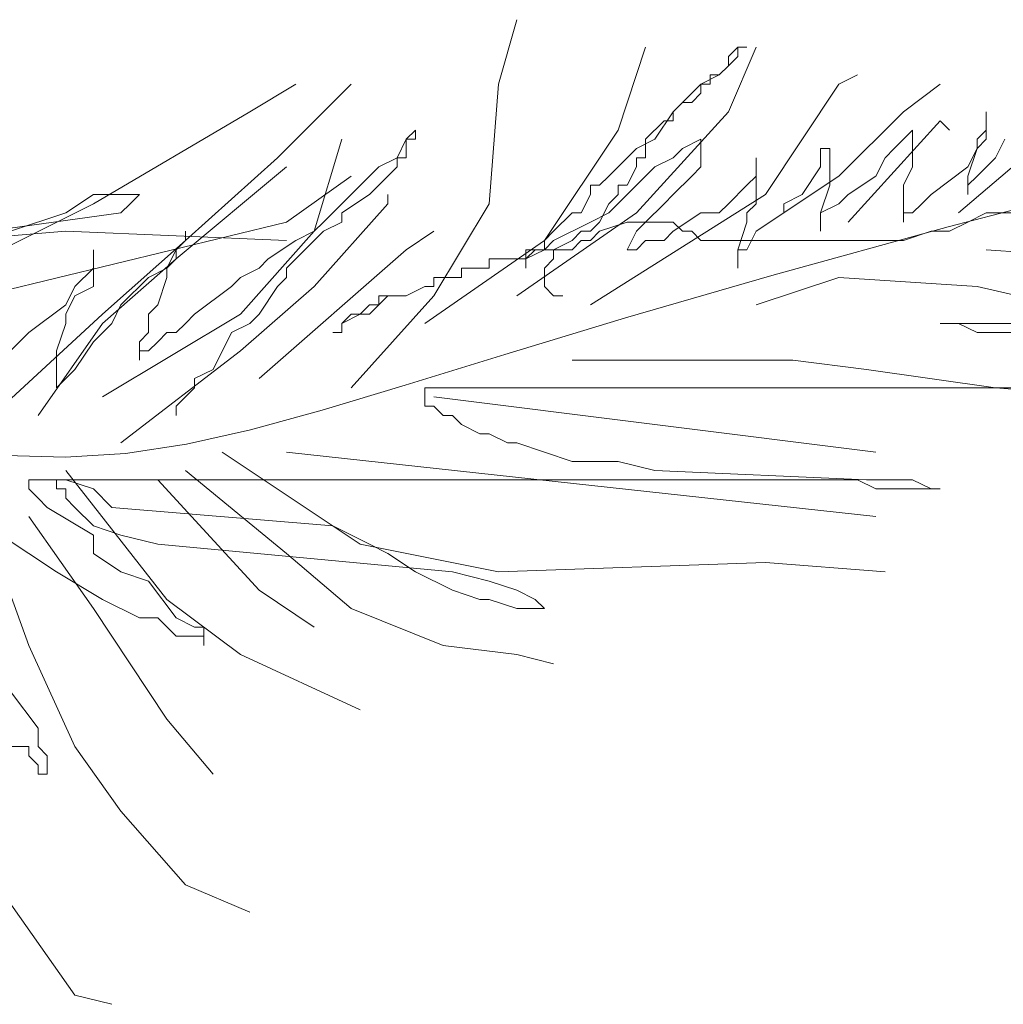
# Model space of a CAD drawing. Units: millimetres. Extents: x 595116 to 630915, y 909473 to 920225.
# Tile 99 of 134: x 629809.617 to 629812.676, y 919168.213 to 919171.275. Entities that reach past the tile are written whole.
import ezdxf

# ---------------------------------------------------------------- set-up
doc = ezdxf.new("R2010")
doc.units = ezdxf.units.MM
doc.layers.add('L-PLNT', color=85, linetype='Continuous', lineweight=13)

# ---------------------------------------------------------------- blocks, each defined once
blk = doc.blocks.new('A$C4FB75ABC')
for p, q in [((4.22491, 2.05804), (4.24016, 2.11139)), ((4.32405, 2.01993), (4.34693, 2.08853)), ((4.41556, 2.0809), (4.42319, 2.08853)), ((4.41556, 2.03517), (4.43844, 2.08853)), ((4.42319, 2.08853), (4.43082, 2.08853)), ((4.43082, 2.08853), (4.42319, 2.08853)), ((4.42319, 2.08853), (4.42319, 2.0809)), ((4.41556, 2.07328), (4.41556, 2.0809)), ((4.42319, 2.0809), (4.41556, 2.07328)), ((4.40794, 2.06566), (4.41556, 2.07328)), ((4.41556, 2.07328), (4.40794, 2.06566)), ((4.40794, 2.06566), (4.39269, 2.05804)), ((4.40031, 2.05804), (4.40031, 2.06566)), ((4.40031, 2.06566), (4.40794, 2.06566)), ((4.50708, 2.05804), (4.52233, 2.06566)), ((4.019, 2.03517), (4.05713, 2.05804)), ((4.04188, 1.99706), (4.10289, 2.05804)), ((4.21728, 1.95895), (4.22491, 2.05804)), ((4.39269, 2.05804), (4.38506, 2.05042)), ((4.39269, 2.05042), (4.39269, 2.05804)), ((4.39269, 2.05804), (4.40031, 2.05804)), ((4.44607, 1.96657), (4.50708, 2.05804)), ((4.56046, 2.03517), (4.59097, 2.05804)), ((4.38506, 2.05042), (4.37743, 2.04279)), ((4.38506, 2.04279), (4.39269, 2.05042)), ((4.36981, 2.03517), (4.37743, 2.04279)), ((4.37743, 2.04279), (4.36981, 2.03517)), ((4.37743, 2.04279), (4.38506, 2.04279)), ((3.88936, 1.95895), (4.019, 2.03517)), ((4.3393, 1.95132), (4.41556, 2.03517)), ((4.36981, 2.03517), (4.35455, 2.0123)), ((4.36981, 2.02755), (4.36981, 2.03517)), ((4.50708, 1.98181), (4.56046, 2.03517)), ((4.6291, 2.01993), (4.6291, 2.03517)), ((4.6291, 2.03517), (4.6291, 2.0123)), ((4.34693, 2.0123), (4.36218, 2.02755)), ((4.36218, 2.02755), (4.36981, 2.02755)), ((4.5147, 1.9437), (4.59097, 2.02755)), ((4.59097, 2.02755), (4.59859, 2.01993)), ((4.15627, 2.01993), (4.14865, 2.0123)), ((4.15627, 2.0123), (4.15627, 2.01993)), ((4.26304, 1.92846), (4.32405, 2.01993)), ((4.56046, 2.0123), (4.56809, 2.01993)), ((4.56809, 2.01993), (4.56809, 1.98944)), ((4.62147, 2.0123), (4.6291, 2.01993)), ((4.07238, 1.93608), (4.09526, 2.0123)), ((4.14865, 2.0123), (4.14102, 1.99706)), ((4.14865, 1.99706), (4.14865, 2.0123)), ((4.14865, 2.0123), (4.15627, 2.0123)), ((4.35455, 2.0123), (4.3393, 2.00468)), ((4.34693, 1.99706), (4.34693, 2.0123)), ((4.37743, 2.00468), (4.39269, 2.0123)), ((4.39269, 2.0123), (4.39269, 1.98944)), ((4.55284, 2.00468), (4.56046, 2.0123)), ((4.62147, 2.00468), (4.62147, 2.0123)), ((4.6291, 2.0123), (4.62147, 2.00468)), ((4.63672, 1.99706), (4.64435, 2.0123)), ((4.3393, 2.00468), (4.33168, 1.99706)), ((4.36981, 1.99706), (4.37743, 2.00468)), ((4.49183, 1.98944), (4.49183, 2.00468)), ((4.49183, 2.00468), (4.49945, 2.00468)), ((4.49945, 2.00468), (4.49945, 1.97419)), ((4.54521, 1.99706), (4.55284, 2.00468)), ((4.61385, 1.98944), (4.62147, 2.00468)), ((4.62147, 2.00468), (4.61385, 1.98181)), ((3.96562, 1.92846), (4.04188, 1.99706)), ((4.14102, 1.99706), (4.12577, 1.98944)), ((4.14102, 1.98944), (4.14102, 1.99706)), ((4.14102, 1.99706), (4.14865, 1.99706)), ((4.33168, 1.99706), (4.31642, 1.98181)), ((4.3393, 1.98944), (4.3393, 1.99706)), ((4.3393, 1.99706), (4.34693, 1.99706)), ((4.35455, 1.98944), (4.36981, 1.99706)), ((4.43844, 1.98181), (4.43844, 1.99706)), ((4.43844, 1.99706), (4.43844, 1.95895)), ((4.53758, 1.98181), (4.54521, 1.99706)), ((4.60622, 1.95132), (4.6596, 1.99706)), ((4.62147, 1.98181), (4.63672, 1.99706)), ((3.95799, 1.91321), (4.04951, 1.98944)), ((4.12577, 1.98944), (4.11814, 1.98181)), ((4.13339, 1.98181), (4.14102, 1.98944)), ((4.33168, 1.97419), (4.3393, 1.98944)), ((4.34693, 1.98181), (4.35455, 1.98944)), ((4.39269, 1.98944), (4.38506, 1.98181)), ((4.47657, 1.96657), (4.49183, 1.98944)), ((4.56809, 1.98944), (4.56046, 1.97419)), ((4.58334, 1.96657), (4.61385, 1.98944)), ((4.77249, 1.98507), (4.5975, 1.93975)), ((4.04951, 1.9437), (4.10289, 1.98181)), ((4.11814, 1.98181), (4.10289, 1.96657)), ((4.11814, 1.96657), (4.13339, 1.98181)), ((4.3088, 1.97419), (4.30117, 1.97419)), ((4.30117, 1.97419), (4.30117, 1.96657)), ((4.31642, 1.98181), (4.3088, 1.97419)), ((4.31642, 1.95132), (4.34693, 1.98181)), ((4.32405, 1.96657), (4.32405, 1.97419)), ((4.32405, 1.97419), (4.33168, 1.97419)), ((4.38506, 1.98181), (4.36981, 1.96657)), ((4.41556, 1.95895), (4.43082, 1.97419)), ((4.43082, 1.97419), (4.43844, 1.98181)), ((4.43844, 1.93608), (4.50708, 1.98181)), ((4.49945, 1.97419), (4.49183, 1.95132)), ((4.5147, 1.96657), (4.53758, 1.98181)), ((4.56046, 1.97419), (4.56046, 1.9437)), ((4.61385, 1.98181), (4.61385, 1.96657)), ((4.61385, 1.97419), (4.62147, 1.98181)), ((4.61385, 1.96657), (4.61385, 1.97419)), ((3.88936, 1.96657), (3.86648, 1.95132)), ((3.92749, 1.96657), (3.88936, 1.96657)), ((3.91986, 1.95895), (3.92749, 1.96657)), ((4.10289, 1.96657), (4.08001, 1.9437)), ((4.09526, 1.95132), (4.11814, 1.96657)), ((4.13339, 1.95895), (4.13339, 1.96657)), ((4.30117, 1.96657), (4.29355, 1.95132)), ((4.30117, 1.8751), (4.44607, 1.96657)), ((4.31642, 1.95895), (4.32405, 1.96657)), ((4.36981, 1.96657), (4.36218, 1.95895)), ((4.46132, 1.95895), (4.47657, 1.96657)), ((4.50708, 1.95895), (4.5147, 1.96657)), ((4.57572, 1.95895), (4.58334, 1.96657)), ((3.75208, 1.89035), (3.88936, 1.95895)), ((3.91223, 1.95132), (3.91986, 1.95895)), ((4.07238, 1.89035), (4.13339, 1.95895)), ((4.17153, 1.88272), (4.21728, 1.95895)), ((4.3088, 1.9437), (4.31642, 1.95895)), ((4.36218, 1.95895), (4.34693, 1.9437)), ((4.40794, 1.95132), (4.41556, 1.95895)), ((4.43844, 1.95895), (4.43082, 1.95132)), ((4.46132, 1.95132), (4.46132, 1.95895)), ((4.49183, 1.95132), (4.50708, 1.95895)), ((4.56809, 1.95132), (4.57572, 1.95895)), ((3.74446, 1.92846), (3.91223, 1.95132)), ((3.86648, 1.95132), (3.82072, 1.93608)), ((4.09526, 1.9437), (4.09526, 1.95132)), ((4.24016, 1.88272), (4.3393, 1.95132)), ((4.28592, 1.95132), (4.27067, 1.93608)), ((4.29355, 1.95132), (4.28592, 1.95132)), ((4.30117, 1.9437), (4.31642, 1.95132)), ((4.36981, 1.93608), (4.39269, 1.95132)), ((4.39269, 1.95132), (4.40794, 1.95132)), ((4.43082, 1.95132), (4.43082, 1.9437)), ((4.43844, 1.93608), (4.46132, 1.95132)), ((4.49183, 1.95132), (4.49183, 1.93608)), ((4.49183, 1.93608), (4.49183, 1.95132)), ((4.56046, 1.95132), (4.56809, 1.95132)), ((4.56046, 1.9437), (4.56046, 1.95132)), ((4.6291, 1.95132), (4.61385, 1.9437)), ((4.65198, 1.95132), (4.6291, 1.95132)), ((3.79784, 1.88272), (4.04951, 1.9437)), ((4.08001, 1.9437), (4.07238, 1.93608)), ((4.08001, 1.93608), (4.09526, 1.9437)), ((4.27067, 1.92846), (4.30117, 1.9437)), ((4.30117, 1.93608), (4.3088, 1.9437)), ((4.33168, 1.9437), (4.3088, 1.93608)), ((4.36981, 1.9437), (4.33168, 1.9437)), ((4.34693, 1.9437), (4.3393, 1.93608)), ((4.37743, 1.93608), (4.36981, 1.9437)), ((4.43082, 1.9437), (4.42319, 1.92083)), ((4.61385, 1.9437), (4.59859, 1.93608)), ((3.58431, 1.91321), (3.86648, 1.93608)), ((3.86648, 1.93608), (4.04951, 1.92846)), ((3.96562, 1.92846), (3.96562, 1.93608)), ((3.96562, 1.93608), (3.96562, 1.92846)), ((4.01138, 1.86748), (4.07238, 1.93608)), ((4.07238, 1.93608), (4.05713, 1.92846)), ((4.07238, 1.92846), (4.08001, 1.93608)), ((4.14865, 1.92083), (4.17153, 1.93608)), ((4.27067, 1.93608), (4.26304, 1.92846)), ((4.28592, 1.92846), (4.29355, 1.93608)), ((4.29355, 1.93608), (4.30117, 1.93608)), ((4.3088, 1.93608), (4.30117, 1.92846)), ((4.3393, 1.93608), (4.33168, 1.92083)), ((4.36218, 1.92846), (4.36981, 1.93608)), ((4.38506, 1.93608), (4.37743, 1.93608)), ((4.39269, 1.92846), (4.38506, 1.93608)), ((4.43082, 1.92083), (4.43844, 1.93608)), ((4.5975, 1.93975), (4.45134, 1.89957)), ((4.58334, 1.93608), (4.56046, 1.92846)), ((4.59859, 1.93608), (4.58334, 1.93608)), ((3.89698, 1.86748), (3.96562, 1.92846)), ((3.95799, 1.92083), (3.96562, 1.92846)), ((3.96562, 1.92846), (3.95799, 1.92083)), ((4.05713, 1.92846), (4.03425, 1.91321)), ((4.05713, 1.91321), (4.07238, 1.92846)), ((4.1639, 1.85986), (4.26304, 1.92846)), ((4.26304, 1.92846), (4.26304, 1.92083)), ((4.26304, 1.92083), (4.27067, 1.92846)), ((4.27067, 1.92083), (4.28592, 1.92846)), ((4.29355, 1.92846), (4.28592, 1.92083)), ((4.30117, 1.92846), (4.29355, 1.92846)), ((4.3393, 1.92083), (4.34693, 1.92846)), ((4.34693, 1.92846), (4.36218, 1.92846)), ((4.56046, 1.92846), (4.39269, 1.92846)), ((3.88936, 1.89035), (3.88936, 1.92083)), ((3.88936, 1.92083), (3.88936, 1.90559)), ((3.95799, 1.92083), (3.95037, 1.90559)), ((3.95799, 1.91321), (3.95799, 1.92083)), ((4.02663, 1.81412), (4.14865, 1.92083)), ((4.25541, 1.92083), (4.24779, 1.91321)), ((4.24779, 1.90559), (4.24779, 1.92083)), ((4.24779, 1.92083), (4.26304, 1.92083)), ((4.26304, 1.92083), (4.24779, 1.91321)), ((4.26304, 1.92083), (4.25541, 1.92083)), ((4.28592, 1.92083), (4.26304, 1.92083)), ((4.27067, 1.91321), (4.27067, 1.92083)), ((4.33168, 1.92083), (4.3393, 1.92083)), ((4.42319, 1.92083), (4.42319, 1.90559)), ((4.42319, 1.90559), (4.42319, 1.92083)), ((4.42319, 1.92083), (4.43082, 1.92083)), ((4.6291, 1.92083), (4.73587, 1.91321)), ((3.89698, 1.85986), (3.95799, 1.91321)), ((3.95037, 1.90559), (3.95799, 1.91321)), ((4.03425, 1.91321), (4.02663, 1.90559)), ((4.04951, 1.90559), (4.05713, 1.91321)), ((4.24779, 1.91321), (4.21728, 1.91321)), ((4.21728, 1.91321), (4.21728, 1.90559)), ((4.24779, 1.91321), (4.24779, 1.90559)), ((4.26304, 1.90559), (4.27067, 1.91321)), ((3.88936, 1.90559), (3.8741, 1.89035)), ((3.95037, 1.90559), (3.93511, 1.89797)), ((3.95037, 1.89797), (3.95037, 1.90559)), ((4.02663, 1.90559), (4.01138, 1.89797)), ((4.04951, 1.89797), (4.04951, 1.90559)), ((4.21728, 1.90559), (4.1944, 1.90559)), ((4.1944, 1.90559), (4.1944, 1.89797)), ((4.26304, 1.89035), (4.26304, 1.90559)), ((3.93511, 1.89797), (3.91223, 1.8751)), ((3.94274, 1.8751), (3.95037, 1.89797)), ((4.01138, 1.89797), (4.00375, 1.89035)), ((4.04188, 1.89035), (4.04951, 1.89797)), ((4.1944, 1.89797), (4.17153, 1.89797)), ((4.17153, 1.89797), (4.17153, 1.89035)), ((4.45134, 1.89957), (4.33019, 1.86441)), ((4.43844, 1.8751), (4.50708, 1.89797)), ((4.50708, 1.89797), (4.62147, 1.89035)), ((3.8741, 1.89035), (3.86648, 1.8751)), ((3.8741, 1.88272), (3.88936, 1.89035)), ((4.00375, 1.89035), (3.97324, 1.86748)), ((4.01138, 1.83699), (4.07238, 1.89035)), ((4.02663, 1.86748), (4.04188, 1.89035)), ((4.1639, 1.89035), (4.14865, 1.88272)), ((4.17153, 1.89035), (4.1639, 1.89035)), ((4.27067, 1.88272), (4.26304, 1.89035)), ((4.62147, 1.89035), (4.72061, 1.86748)), ((3.86648, 1.86748), (3.8741, 1.88272)), ((4.10289, 1.8065), (4.17153, 1.88272)), ((4.13339, 1.88272), (4.12577, 1.8751)), ((4.12577, 1.8751), (4.12577, 1.88272)), ((4.12577, 1.88272), (4.13339, 1.88272)), ((4.14865, 1.88272), (4.13339, 1.88272)), ((4.27829, 1.88272), (4.27067, 1.88272)), ((3.86648, 1.8751), (3.83597, 1.85223)), ((3.91223, 1.8751), (3.90461, 1.85986)), ((3.93511, 1.86748), (3.94274, 1.8751)), ((4.11814, 1.8751), (4.11052, 1.86748)), ((4.12577, 1.8751), (4.11814, 1.8751)), ((4.11814, 1.86748), (4.12577, 1.8751)), ((3.79784, 1.77601), (3.89698, 1.86748)), ((3.8436, 1.78363), (3.89698, 1.85986)), ((3.85885, 1.83699), (3.86648, 1.85986)), ((3.86648, 1.85986), (3.86648, 1.86748)), ((3.90461, 1.85986), (3.88936, 1.84461)), ((3.89698, 1.79888), (4.01138, 1.86748)), ((3.93511, 1.85223), (3.93511, 1.86748)), ((3.96562, 1.85986), (3.95799, 1.85223)), ((3.97324, 1.86748), (3.96562, 1.85986)), ((4.00375, 1.85223), (4.019, 1.85986)), ((4.019, 1.85986), (4.02663, 1.86748)), ((4.10289, 1.86748), (4.09526, 1.85986)), ((4.09526, 1.85986), (4.11052, 1.86748)), ((4.09526, 1.85986), (4.09526, 1.85223)), ((4.09526, 1.85223), (4.09526, 1.85986)), ((4.11052, 1.86748), (4.10289, 1.86748)), ((4.11052, 1.86748), (4.11814, 1.86748)), ((4.33019, 1.86441), (4.23027, 1.83415)), ((4.60622, 1.85986), (4.59097, 1.85986)), ((4.59097, 1.85986), (4.65198, 1.85986)), ((4.62147, 1.85223), (4.60622, 1.85986)), ((3.83597, 1.85223), (3.82072, 1.83699)), ((3.92749, 1.84461), (3.93511, 1.85223)), ((3.95037, 1.85223), (3.94274, 1.84461)), ((3.95799, 1.85223), (3.95037, 1.85223)), ((3.9885, 1.82174), (4.00375, 1.85223)), ((4.09526, 1.85223), (4.08764, 1.85223)), ((4.08764, 1.85223), (4.09526, 1.85223)), ((4.67486, 1.85223), (4.62147, 1.85223)), ((3.88936, 1.84461), (3.8741, 1.82174)), ((3.92749, 1.82937), (3.92749, 1.84461)), ((3.94274, 1.84461), (3.93511, 1.83699)), ((3.85885, 1.8065), (3.85885, 1.83699)), ((3.91223, 1.76077), (4.01138, 1.83699)), ((3.93511, 1.83699), (3.92749, 1.83699)), ((3.92749, 1.83699), (3.92749, 1.82937)), ((4.23027, 1.83415), (4.14774, 1.80866)), ((4.28592, 1.82937), (4.46895, 1.82937)), ((4.46895, 1.82937), (4.52996, 1.82174)), ((3.8741, 1.82174), (3.86648, 1.81412)), ((3.97324, 1.81412), (3.9885, 1.82174)), ((4.52996, 1.82174), (4.63672, 1.8065)), ((3.86648, 1.81412), (3.85885, 1.8065)), ((3.97324, 1.8065), (3.97324, 1.81412)), ((3.96562, 1.79888), (3.97324, 1.8065)), ((4.14774, 1.80866), (4.07882, 1.78783)), ((4.1639, 1.79125), (4.1639, 1.8065)), ((4.1639, 1.8065), (5.03329, 1.8065)), ((4.63672, 1.8065), (4.73587, 1.79888)), ((3.95799, 1.79125), (3.96562, 1.79888)), ((4.17153, 1.79888), (4.53758, 1.75314)), ((3.95799, 1.78363), (3.95799, 1.79125)), ((4.07882, 1.78783), (4.01969, 1.77155)), ((4.17153, 1.79125), (4.1639, 1.79125)), ((4.17915, 1.78363), (4.17153, 1.79125)), ((4.18678, 1.78363), (4.17915, 1.78363)), ((4.1944, 1.77601), (4.18678, 1.78363)), ((4.01969, 1.77155), (3.96655, 1.75968)), ((4.20966, 1.76839), (4.1944, 1.77601)), ((4.21728, 1.76839), (4.20966, 1.76839)), ((4.23254, 1.76077), (4.21728, 1.76839)), ((3.96655, 1.75968), (3.91602, 1.75215)), ((4.24016, 1.76077), (4.23254, 1.76077)), ((4.28592, 1.74552), (4.24016, 1.76077)), ((3.86643, 1.74902), (3.81654, 1.75042)), ((3.91602, 1.75215), (3.86643, 1.74902)), ((3.99612, 1.75314), (4.11052, 1.67692)), ((4.04951, 1.75314), (4.53758, 1.69979)), ((4.32405, 1.74552), (4.28592, 1.74552)), ((4.35455, 1.7379), (4.32405, 1.74552)), ((3.86648, 1.7379), (3.95037, 1.63118)), ((3.96562, 1.7379), (4.04951, 1.6693)), ((4.52996, 1.73028), (4.35455, 1.7379)), ((3.83597, 1.72265), (3.83597, 1.73028)), ((3.83597, 1.73028), (3.86648, 1.73028)), ((3.85885, 1.72265), (3.85885, 1.73028)), ((3.85885, 1.73028), (4.52233, 1.73028)), ((3.86648, 1.73028), (3.88936, 1.72265)), ((3.94274, 1.73028), (4.02663, 1.63881)), ((4.52233, 1.73028), (4.53758, 1.72265)), ((4.56809, 1.73028), (4.52996, 1.73028)), ((4.58334, 1.72265), (4.56809, 1.73028)), ((3.8436, 1.71503), (3.83597, 1.72265)), ((3.86648, 1.72265), (3.85885, 1.72265)), ((3.86648, 1.71503), (3.86648, 1.72265)), ((3.88936, 1.72265), (3.90461, 1.70741)), ((4.53758, 1.72265), (4.59097, 1.72265)), ((4.59097, 1.72265), (4.58334, 1.72265)), ((3.85122, 1.70741), (3.8436, 1.71503)), ((3.8741, 1.70741), (3.86648, 1.71503)), ((3.88936, 1.68454), (3.85122, 1.70741)), ((3.88936, 1.69216), (3.8741, 1.70741)), ((3.90461, 1.70741), (4.08764, 1.69216)), ((3.83597, 1.69979), (3.88936, 1.62356)), ((3.91223, 1.68454), (3.88936, 1.69216)), ((4.08764, 1.69216), (4.11814, 1.67692)), ((3.81309, 1.68454), (3.83597, 1.6693)), ((3.88936, 1.6693), (3.88936, 1.68454)), ((3.94274, 1.67692), (3.91223, 1.68454)), ((3.80547, 1.67692), (3.83597, 1.59307)), ((4.18678, 1.65405), (3.94274, 1.67692)), ((4.11052, 1.67692), (4.22491, 1.65405)), ((4.11814, 1.67692), (4.13339, 1.6693)), ((3.83597, 1.6693), (3.85885, 1.65405)), ((3.91223, 1.65405), (3.88936, 1.6693)), ((4.04951, 1.6693), (4.10289, 1.62356)), ((4.13339, 1.6693), (4.15627, 1.65405)), ((4.22491, 1.65405), (4.44607, 1.66167)), ((4.44607, 1.66167), (4.54521, 1.65405)), ((3.85885, 1.65405), (3.89698, 1.63118)), ((3.93511, 1.64643), (3.91223, 1.65405)), ((4.15627, 1.65405), (4.18678, 1.63881)), ((4.21728, 1.64643), (4.18678, 1.65405)), ((3.95799, 1.61594), (3.93511, 1.64643)), ((4.24016, 1.63881), (4.21728, 1.64643)), ((4.02663, 1.63881), (4.07238, 1.60832)), ((4.18678, 1.63881), (4.20966, 1.63118)), ((4.25541, 1.63118), (4.24016, 1.63881)), ((3.88936, 1.62356), (3.95037, 1.53209)), ((3.89698, 1.63118), (3.92749, 1.61594)), ((3.95037, 1.63118), (4.01138, 1.58545)), ((4.10289, 1.62356), (4.17915, 1.59307)), ((4.20966, 1.63118), (4.21728, 1.63118)), ((4.21728, 1.63118), (4.24016, 1.62356)), ((4.24016, 1.62356), (4.26304, 1.62356)), ((4.26304, 1.62356), (4.25541, 1.63118)), ((3.92749, 1.61594), (3.94274, 1.61594)), ((3.94274, 1.61594), (3.95799, 1.6007)), ((3.97324, 1.60832), (3.95799, 1.61594)), ((3.98087, 1.60832), (3.97324, 1.60832)), ((3.98087, 1.59307), (3.98087, 1.60832)), ((3.95799, 1.6007), (3.98087, 1.6007)), ((3.98087, 1.6007), (3.98087, 1.59307)), ((3.83597, 1.59307), (3.8741, 1.50923)), ((4.17915, 1.59307), (4.24016, 1.58545)), ((4.01138, 1.58545), (4.11052, 1.53972)), ((4.24016, 1.58545), (4.27067, 1.57783)), ((3.8436, 1.52447), (3.82072, 1.55496)), ((3.95037, 1.53209), (3.9885, 1.48636)), ((3.8436, 1.50923), (3.8436, 1.52447)), ((3.82072, 1.50923), (3.83597, 1.50923)), ((3.83597, 1.50923), (3.83597, 1.50161)), ((3.85122, 1.50161), (3.8436, 1.50923)), ((3.8741, 1.50923), (3.91223, 1.45587)), ((3.83597, 1.50161), (3.8436, 1.49398)), ((3.85122, 1.48636), (3.85122, 1.50161)), ((3.8436, 1.49398), (3.8436, 1.48636)), ((3.8436, 1.48636), (3.85122, 1.48636)), ((3.91223, 1.45587), (3.96562, 1.39489)), ((3.78259, 1.433), (3.8741, 1.30342)), ((3.96562, 1.39489), (4.019, 1.37203)), ((3.8741, 1.30342), (3.90461, 1.2958))]:
    blk.add_line(p, q)

msp = doc.modelspace()

# ---------------------------------------------------------------- block references
at = {"layer": 'L-PLNT', "xscale": 3.753413438031968, "yscale": 3.753413438031968, "zscale": 3.753413438031968}
msp.add_blockref('A$C4FB75ABC', (629795.2477, 919163.3497), dxfattribs=at)

doc.saveas('drawing.dxf')
